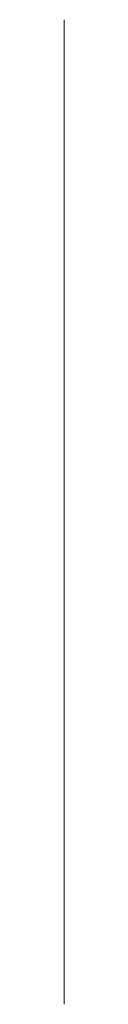
# Model space of a CAD drawing. Units: millimetres. Extents: x 222.15 to 222.15, y 22.5 to 27.5.
import ezdxf

# ---------------------------------------------------------------- set-up
doc = ezdxf.new("R2010")
doc.units = ezdxf.units.MM
doc.layers.add('M-CONS', color=8, linetype='Continuous', lineweight=13)

msp = doc.modelspace()

# ---------------------------------------------------------------- linework, layer by layer
at = {"layer": 'M-CONS', "extrusion": (0, -1, 0)}
msp.add_line((222.1536, 27.5, 392.4934), (222.1536, 22.5, 392.4934), dxfattribs=at)

doc.saveas('drawing.dxf')
